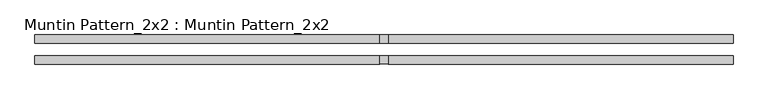
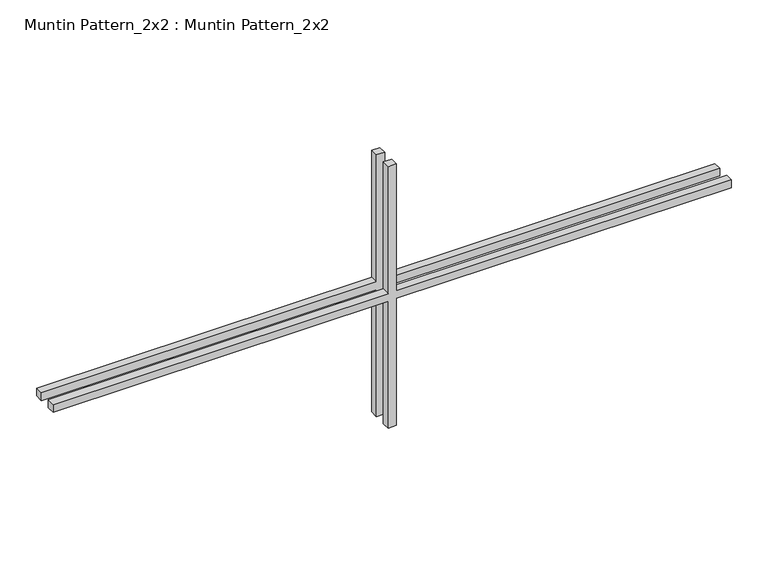
"""IFC4 building model written with IfcOpenShell, lengths in millimetres: proxy geometry, Muntin Pattern_2x2 : Muntin Pattern_2x2."""

from ifc_helpers import new_model, si_unit, frame, origin, place, context, project, spatial, polyline, outline, extrude, source, transform, mapped, element, save


def muntin_pattern_2x2_muntin_pattern_2x2_5e52a1c6(model_context):
    return source(origin(), model_context, "Body", "SweptSolid", [
        extrude(outline(polyline([(223.8375, -6.35), (223.8375, -533.4), (211.1375, -533.4), (211.1375, -6.35), (0.0, -6.35), (0.0, 6.35), (211.1375, 6.35), (211.1375, 533.4), (223.8375, 533.4), (223.8375, 6.35), (434.975, 6.35), (434.975, -6.35), (223.8375, -6.35)])), frame((0.0, -22.225, 0.0), z_axis=(0.0, 1.0, 0.0), x_axis=(0.0, 0.0, 1.0)), (0.0, 0.0, 1.0), 12.7),
        extrude(outline(polyline([(223.8375, -6.35), (223.8375, -533.4), (211.1375, -533.4), (211.1375, -6.35), (0.0, -6.35), (0.0, 6.35), (211.1375, 6.35), (211.1375, 533.4), (223.8375, 533.4), (223.8375, 6.35), (434.975, 6.35), (434.975, -6.35), (223.8375, -6.35)])), frame((0.0, 9.525, 0.0), z_axis=(0.0, 1.0, 0.0), x_axis=(0.0, 0.0, 1.0)), (0.0, 0.0, 1.0), 12.7),
    ])


if __name__ == "__main__":
    model = new_model("IFC4")
    model_context = context("Model", 3, world=origin())
    ifc_project = project(units=[si_unit("LENGTHUNIT", "METRE", prefix="MILLI")], contexts=[model_context])
    site = spatial("IfcSite", under=ifc_project)
    building = spatial("IfcBuilding", under=site)
    placement = place(None, origin())
    muntin_pattern_2x2_muntin_pattern_2x2_shape = muntin_pattern_2x2_muntin_pattern_2x2_5e52a1c6(model_context)
    element("IfcBuildingElementProxy", 1, Name="Muntin Pattern_2x2 : Muntin Pattern_2x2", ObjectType="Muntin Pattern_2x2 : Muntin Pattern_2x2", at=placement, inside=building, context=model_context, shape_type="MappedRepresentation", body=[
        mapped(muntin_pattern_2x2_muntin_pattern_2x2_shape, transform((0.0, 0.0, 0.0), x_axis=(1.0, 0.0, 0.0), y_axis=(0.0, 1.0, 0.0), z_axis=(0.0, 0.0, 1.0))),
    ])
    save(model, "model.ifc")

# Revit data of these elements
# Type "Muntin Pattern_2x2 : Muntin Pattern_2x2"
#   Width [instance default] = 4' - 0"
#   Thickness = 0' - 0 1/2"
#   Height [instance default] = 4' - 0"
#   Distance = 0' - 0 3/4"
#   Interior Material [instance default] = none
#   Exterior Material [instance default] = none
#   Default Elevation = 0
# Element 1 (IfcBuildingElementProxy, "Muntin Pattern_2x2 : Muntin Pattern_2x2")
#   Width = 3' - 6"
#   Height = 1' - 5 1/8"
#   Interior Material = Wood - Stained
#   Exterior Material = Clad - White
#   Materials on its faces: "Clad - White", "Wood - Stained"
# Materials
#   "Clad - White": class "Wood", colour RGB 242 242 238, transparency 0, Cost = 0
#   "Wood - Stained": class "Wood", colour RGB 224 178 126, transparency 0, Cost = 0
